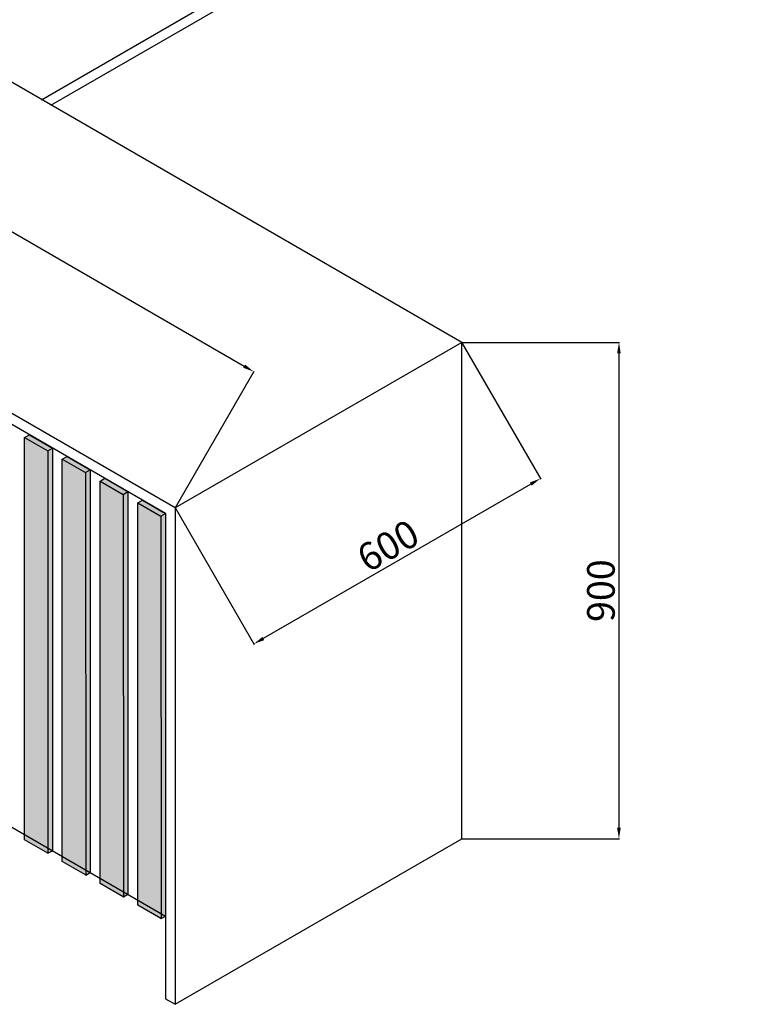
# Model space of a CAD drawing. Units: centimetres. Extents: x 209356 to 217348, y 253987 to 259034.
# Tile 2 of 7: x 210968 to 212290, y 253987 to 255772. Entities that reach past the tile are written whole.
import ezdxf

# ---------------------------------------------------------------- set-up
doc = ezdxf.new("R2010")
doc.units = ezdxf.units.CM
for name, color, linetype, lineweight in [('A-ANNO-DIMS', 2, 'Continuous', 18), ('A-ELEV', 7, 'Continuous', 25), ('A-ELEV-PATT', 32, 'Continuous', 13)]:
    doc.layers.add(name, color=color, linetype=linetype, lineweight=lineweight)
doc.styles.get("Standard").update_dxf_attribs({"font": 'arial.ttf'})
doc.dimstyles.new('ISO-25', dxfattribs={"dimtxt": 50, "dimasz": 20, "dimexe": 1.25, "dimexo": 0.625, "dimtad": 1, "dimdec": 1, "dimtxsty": 'Standard', "dimcen": 2.5, "dimadec": 0, "dimazin": 0, "dimtfac": 1, "dimtdec": 1, "dimtmove": 0, "dimatfit": 3, "dimfxl": 1, "dimarcsym": 0})

# ---------------------------------------------------------------- blocks, each defined once
blk = doc.blocks.new('FLUTED-PANEL')
for p, q in [((0, 753.9), (8.7, 758.9)), ((0, 24.5), (0, 753.9)), ((0, 753.9), (41.9, 729.7)), ((8.7, 758.9), (50.6, 734.7)), ((41.9, 729.7), (50.6, 734.7)), ((50.6, 734.7), (50.6, 4.7)), ((41.9, 729.7), (42.4, 0)), ((41.9, 0.3), (0, 24.5)), ((41.9, 0.3), (42.4, 0)), ((42.4, 0), (50.6, 4.7))]:
    blk.add_line(p, q)
blk = doc.blocks.new('*D12')
at = {"layer": 'A-ANNO-DIMS', "color": 0, "lineweight": -2, "transparency": 16777216}
for p, q in [((209691.8, 255787.1), (209834.6, 256034.4)), ((209851.3, 256023.4), (211375.5, 255143.4)), ((211250.7, 254887.1), (211393.5, 255134.4))]:
    blk.add_line(p, q, dxfattribs=at)
at = {"layer": 'A-ANNO-DIMS', "color": 0, "transparency": 16777216}
for points in [[(209853, 256026.3), (209849.6, 256020.5), (209834, 256033.4)], [(211377.2, 255146.3), (211373.9, 255140.5), (211392.8, 255133.4)]]:
    blk.add_solid(points, dxfattribs=at)
at = {"layer": 'Defpoints', "color": 0, "transparency": 16777216}
for p in [(209691.5, 255786.5), (211392.8, 255133.4), (211250.3, 254886.5)]:
    blk.add_point(p, dxfattribs=at)
at = {"layer": 'A-ANNO-DIMS', "color": 0, "transparency": 16777216, "insert": (210626.5, 255606), "char_height": 50, "attachment_point": 5, "rotation": 330}
blk.add_mtext('1800', dxfattribs=at)
blk = doc.blocks.new('*D13')
at = {"layer": 'A-ANNO-DIMS', "color": 0, "lineweight": -2, "transparency": 16777216}
for p, q in [((211770.3, 255186), (211913.1, 254938.6)), ((211895.1, 254929.7), (211410.2, 254649.7)), ((211250.7, 254886), (211393.5, 254638.6))]:
    blk.add_line(p, q, dxfattribs=at)
at = {"layer": 'A-ANNO-DIMS', "color": 0, "transparency": 16777216}
for points in [[(211893.5, 254932.6), (211896.8, 254926.8), (211912.5, 254939.7)], [(211408.5, 254652.6), (211411.8, 254646.8), (211392.8, 254639.7)]]:
    blk.add_solid(points, dxfattribs=at)
at = {"layer": 'Defpoints', "color": 0, "transparency": 16777216}
for p in [(211770, 255186.5), (211250.3, 254886.5), (211392.8, 254639.7)]:
    blk.add_point(p, dxfattribs=at)
at = {"layer": 'A-ANNO-DIMS', "color": 0, "transparency": 16777216, "insert": (211639.6, 254812.4), "char_height": 50, "attachment_point": 5, "rotation": 30}
blk.add_mtext('600', dxfattribs=at)
blk = doc.blocks.new('*D14')
at = {"layer": 'A-ANNO-DIMS', "color": 0, "lineweight": -2, "transparency": 16777216}
for p, q in [((211770.6, 255186.5), (212056.2, 255186.5)), ((212055, 255166.5), (212055, 254306.5)), ((211770.6, 254286.5), (212056.2, 254286.5))]:
    blk.add_line(p, q, dxfattribs=at)
at = {"layer": 'A-ANNO-DIMS', "color": 0, "transparency": 16777216}
for points in [[(212051.6, 255166.5), (212058.3, 255166.5), (212055, 255186.5)], [(212051.6, 254306.5), (212058.3, 254306.5), (212055, 254286.5)]]:
    blk.add_solid(points, dxfattribs=at)
at = {"layer": 'Defpoints', "color": 0, "transparency": 16777216}
for p in [(211770, 255186.5), (211770, 254286.5), (212055, 254286.5)]:
    blk.add_point(p, dxfattribs=at)
at = {"layer": 'A-ANNO-DIMS', "color": 0, "transparency": 16777216, "insert": (212028.8, 254736.5), "char_height": 50, "attachment_point": 5, "rotation": 90}
blk.add_mtext('900', dxfattribs=at)

msp = doc.modelspace()

# ---------------------------------------------------------------- hatches: boundary and pattern name
at = {"layer": 'A-ELEV-PATT'}
h = msp.add_hatch(color=256, dxfattribs=at)
h.dxf.hatch_style = 1
h.paths.add_polyline_path([(210985.9821, 255019.1753), (210977.3288, 255014.1793), (211019.2445, 254989.9792), (211027.8978, 254994.9752)])
h.paths.add_polyline_path([(211019.7514, 254260.2719), (211027.8978, 254264.9752), (211027.8978, 254994.9752), (211019.2445, 254989.9792)])
h.paths.add_polyline_path([(210977.3288, 254284.7646), (211019.7514, 254260.2719), (211019.2445, 254989.9792), (210977.3288, 255014.1793)])
h = msp.add_hatch(color=256, dxfattribs=at)
h.dxf.hatch_style = 1
h.paths.add_polyline_path([(211054.3554, 254979.6999), (211045.7021, 254974.7039), (211087.6178, 254950.5039), (211096.2711, 254955.4999)])
h.paths.add_polyline_path([(211088.1248, 254220.7965), (211096.2711, 254225.4999), (211096.2711, 254955.4999), (211087.6178, 254950.5039)])
h.paths.add_polyline_path([(211045.7021, 254245.2893), (211088.1248, 254220.7965), (211087.6178, 254950.5039), (211045.7021, 254974.7039)])
h = msp.add_hatch(color=256, dxfattribs=at)
h.dxf.hatch_style = 1
h.paths.add_polyline_path([(211122.7287, 254940.2246), (211114.0754, 254935.2286), (211155.9912, 254911.0285), (211164.6445, 254916.0245)])
h.paths.add_polyline_path([(211156.4981, 254181.3212), (211164.6445, 254186.0245), (211164.6445, 254916.0245), (211155.9912, 254911.0285)])
h.paths.add_polyline_path([(211114.0754, 254205.8139), (211156.4981, 254181.3212), (211155.9912, 254911.0285), (211114.0754, 254935.2286)])
h = msp.add_hatch(color=256, dxfattribs=at)
h.dxf.hatch_style = 1
h.paths.add_polyline_path([(211191.1021, 254900.7492), (211182.4487, 254895.7532), (211224.3645, 254871.5532), (211233.0178, 254876.5492)])
h.paths.add_polyline_path([(211224.8714, 254141.8458), (211233.0178, 254146.5492), (211233.0178, 254876.5492), (211224.3645, 254871.5532)])
h.paths.add_polyline_path([(211182.4487, 254166.3386), (211224.8714, 254141.8458), (211224.3645, 254871.5532), (211182.4487, 254895.7532)])

# ---------------------------------------------------------------- linework, layer by layer
at = {"layer": 'A-ELEV'}
for p, q in [((211007.8512, 255626.5492), (212289.5688, 256366.5492)), ((211025.1717, 255616.5492), (212289.5688, 256346.5492)), ((211769.9535, 255186.5492), (210211.1078, 256086.5492)), ((211250.3383, 254886.5492), (209691.4926, 255786.5492)), ((211233.0178, 254876.5492), (209691.4926, 255766.5492)), ((211769.9535, 255186.5492), (211250.3383, 254886.5492)), ((211769.9535, 254286.5492), (211769.9535, 255186.5492)), ((211182.4487, 254895.7532), (211191.1021, 254900.7492)), ((211191.1021, 254900.7492), (211233.0178, 254876.5492)), ((211182.4487, 254166.3386), (211182.4487, 254895.7532)), ((211182.4487, 254895.7532), (211224.3645, 254871.5532)), ((211250.3383, 254886.5492), (211250.3383, 253986.5492)), ((211224.3645, 254871.5532), (211233.0178, 254876.5492)), ((211224.3645, 254871.5532), (211224.8714, 254141.8458)), ((211233.0178, 254876.5492), (211233.0178, 253996.5492)), ((211233.0178, 254876.5492), (211233.0178, 254146.5492)), ((210491.2201, 254574.8262), (211233.0178, 254146.5492)), ((211250.3383, 253986.5492), (211769.9535, 254286.5492)), ((211224.3645, 254142.1385), (211182.4487, 254166.3386)), ((211224.3645, 254142.1385), (211224.8714, 254141.8458)), ((211224.8714, 254141.8458), (211233.0178, 254146.5492)), ((211233.0178, 253996.5492), (211250.3383, 253986.5492))]:
    msp.add_line(p, q, dxfattribs=at)

# ---------------------------------------------------------------- block references
for p in [(210977.3284, 254260.2717), (211045.7017, 254220.7964), (211114.075, 254181.321)]:
    msp.add_blockref('FLUTED-PANEL', p, dxfattribs=at)

# ---------------------------------------------------------------- dimensions: what is measured, and where the dimension line sits
at = {"layer": 'A-ANNO-DIMS'}
for base, p1, p2, angle, picture, middle in [((211392.8383, 255133.3664), (209691.4926, 255786.5492), (211250.3383, 254886.5492), 330, '*D12', (210626.4923, 255606.0161)), ((211392.8383, 254639.7319), (211769.9535, 255186.5492), (211250.3383, 254886.5492), 210, '*D13', (211639.5691, 254812.3816)), ((212054.9535, 254286.5492), (211769.9535, 255186.5492), (211769.9535, 254286.5492), 270, '*D14', (212028.7999, 254736.5492))]:
    dim = msp.add_linear_dim(base=base, p1=p1, p2=p2, angle=angle, dimstyle='ISO-25', override={"dimdec": 0, "dimlfac": 1, "dimrnd": 0, "dimzin": 0, "dimdsep": 46, "dimlunit": 2}, dxfattribs=at)
    dim.commit()
    dim.dimension.update_dxf_attribs({"geometry": picture, "text_midpoint": middle})

doc.saveas('drawing.dxf')
